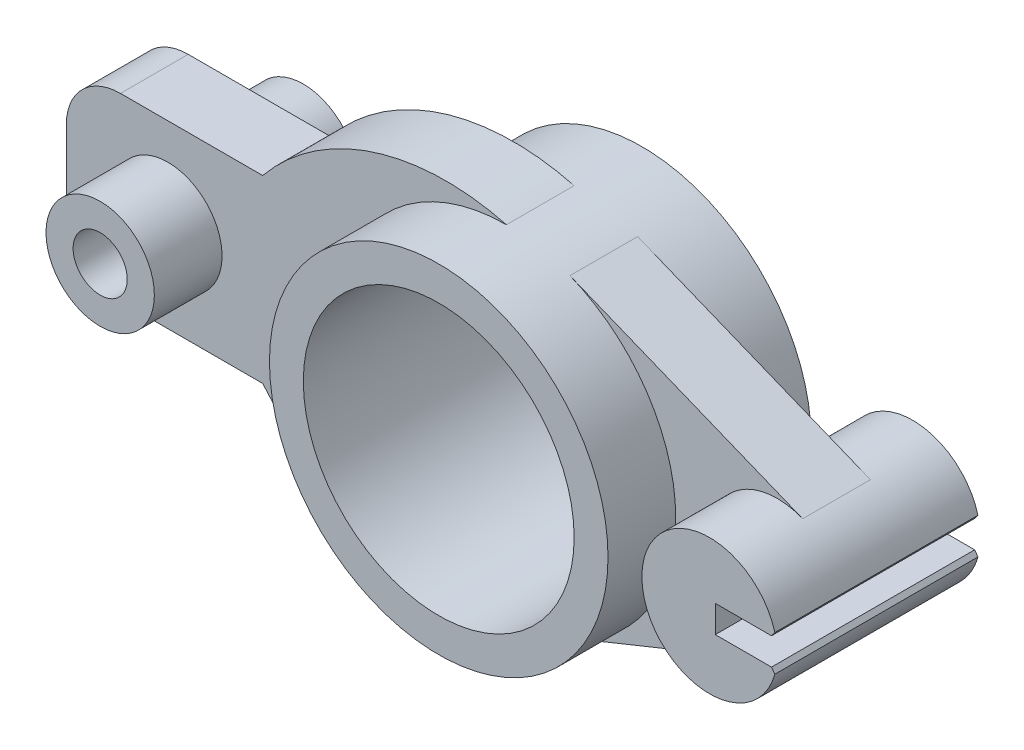
ISO-10303-21;
HEADER;
FILE_DESCRIPTION(('STEP AP214'),'2;1');
FILE_NAME('part.step','',(''),(''),'','','');
FILE_SCHEMA(('AUTOMOTIVE_DESIGN { 1 0 10303 214 1 1 1 1 }'));
ENDSEC;
DATA;
#1=APPLICATION_CONTEXT('core data for automotive mechanical design processes');
#2=APPLICATION_PROTOCOL_DEFINITION('international standard','automotive_design',2000,#1);
#3=PRODUCT_CONTEXT('',#1,'mechanical');
#4=PRODUCT('Part','Part','',(#3));
#5=PRODUCT_RELATED_PRODUCT_CATEGORY('part','',(#4));
#6=PRODUCT_DEFINITION_FORMATION('','',#4);
#7=PRODUCT_DEFINITION_CONTEXT('part definition',#1,'design');
#8=PRODUCT_DEFINITION('design','',#6,#7);
#9=PRODUCT_DEFINITION_SHAPE('','',#8);
#10=(LENGTH_UNIT() NAMED_UNIT(*) SI_UNIT(.MILLI.,.METRE.));
#11=(NAMED_UNIT(*) PLANE_ANGLE_UNIT() SI_UNIT($,.RADIAN.));
#12=(NAMED_UNIT(*) SI_UNIT($,.STERADIAN.) SOLID_ANGLE_UNIT());
#13=UNCERTAINTY_MEASURE_WITH_UNIT(LENGTH_MEASURE(1.E-05),#10,'distance_accuracy_value','');
#14=(GEOMETRIC_REPRESENTATION_CONTEXT(3) GLOBAL_UNCERTAINTY_ASSIGNED_CONTEXT((#13)) GLOBAL_UNIT_ASSIGNED_CONTEXT((#10,
#11,#12)) REPRESENTATION_CONTEXT('',''));
#15=CARTESIAN_POINT('',(0.,0.,0.));
#16=DIRECTION('',(0.,0.,1.));
#17=DIRECTION('',(1.,0.,0.));
#18=AXIS2_PLACEMENT_3D('',#15,#16,#17);
#19=CARTESIAN_POINT('',(0.,0.,15.));
#20=DIRECTION('',(0.,0.,-1.));
#21=DIRECTION('',(-1.,0.,0.));
#22=AXIS2_PLACEMENT_3D('',#19,#20,#21);
#23=CYLINDRICAL_SURFACE('',#22,25.);
#24=CARTESIAN_POINT('',(0.,0.,5.));
#25=DIRECTION('',(0.,0.,-1.));
#26=DIRECTION('',(-1.,0.,0.));
#27=AXIS2_PLACEMENT_3D('',#24,#25,#26);
#28=CIRCLE('',#27,25.);
#29=CARTESIAN_POINT('',(9.37500000000001,23.175620272174,5.));
#30=VERTEX_POINT('',#29);
#31=CARTESIAN_POINT('',(9.37499999999999,-23.175620272174,5.));
#32=VERTEX_POINT('',#31);
#33=EDGE_CURVE('E50',#30,#32,#28,.T.);
#34=ORIENTED_EDGE('',*,*,#33,.F.);
#35=DIRECTION('',(0.,0.,-1.));
#36=VECTOR('',#35,1.);
#37=CARTESIAN_POINT('',(9.37500000000001,23.175620272174,5.));
#38=LINE('',#37,#36);
#39=CARTESIAN_POINT('',(9.37500000000001,23.175620272174,-5.));
#40=VERTEX_POINT('',#39);
#41=EDGE_CURVE('E285',#30,#40,#38,.T.);
#42=ORIENTED_EDGE('',*,*,#41,.T.);
#43=CARTESIAN_POINT('',(0.,0.,-5.));
#44=DIRECTION('',(0.,0.,-1.));
#45=DIRECTION('',(-1.,0.,0.));
#46=AXIS2_PLACEMENT_3D('',#43,#44,#45);
#47=CIRCLE('',#46,25.);
#48=CARTESIAN_POINT('',(9.37500000000001,-23.1756202721739,-5.));
#49=VERTEX_POINT('',#48);
#50=EDGE_CURVE('E323',#40,#49,#47,.T.);
#51=ORIENTED_EDGE('',*,*,#50,.T.);
#52=DIRECTION('',(0.,0.,-1.));
#53=VECTOR('',#52,1.);
#54=CARTESIAN_POINT('',(9.37499999999999,-23.175620272174,5.));
#55=LINE('',#54,#53);
#56=EDGE_CURVE('E295',#32,#49,#55,.T.);
#57=ORIENTED_EDGE('',*,*,#56,.F.);
#58=EDGE_LOOP('',(#34,#42,#51,#57));
#59=FACE_BOUND('',#58,.T.);
#60=CARTESIAN_POINT('',(0.,-25.,-5.));
#61=VERTEX_POINT('',#60);
#62=CARTESIAN_POINT('',(0.,25.,-5.));
#63=VERTEX_POINT('',#62);
#64=EDGE_CURVE('E317',#61,#63,#47,.T.);
#65=ORIENTED_EDGE('',*,*,#64,.T.);
#66=DIRECTION('',(0.,0.,-1.));
#67=VECTOR('',#66,1.);
#68=CARTESIAN_POINT('',(0.,25.,5.));
#69=LINE('',#68,#67);
#70=CARTESIAN_POINT('',(0.,25.,5.));
#71=VERTEX_POINT('',#70);
#72=EDGE_CURVE('E261',#71,#63,#69,.T.);
#73=ORIENTED_EDGE('',*,*,#72,.F.);
#74=CARTESIAN_POINT('',(0.,-25.,5.));
#75=VERTEX_POINT('',#74);
#76=EDGE_CURVE('E322',#75,#71,#28,.T.);
#77=ORIENTED_EDGE('',*,*,#76,.F.);
#78=DIRECTION('',(0.,0.,-1.));
#79=VECTOR('',#78,1.);
#80=CARTESIAN_POINT('',(0.,-25.,5.));
#81=LINE('',#80,#79);
#82=EDGE_CURVE('E294',#75,#61,#81,.T.);
#83=ORIENTED_EDGE('',*,*,#82,.T.);
#84=EDGE_LOOP('',(#65,#73,#77,#83));
#85=FACE_BOUND('',#84,.T.);
#86=CARTESIAN_POINT('',(0.,0.,-15.));
#87=DIRECTION('',(0.,0.,1.));
#88=DIRECTION('',(1.,0.,0.));
#89=AXIS2_PLACEMENT_3D('',#86,#87,#88);
#90=CIRCLE('',#89,25.);
#91=CARTESIAN_POINT('',(25.,0.,-15.));
#92=VERTEX_POINT('',#91);
#93=EDGE_CURVE('E312',#92,#92,#90,.T.);
#94=ORIENTED_EDGE('',*,*,#93,.T.);
#95=EDGE_LOOP('',(#94));
#96=FACE_BOUND('',#95,.T.);
#97=CARTESIAN_POINT('',(0.,0.,15.));
#98=DIRECTION('',(0.,0.,1.));
#99=DIRECTION('',(1.,0.,0.));
#100=AXIS2_PLACEMENT_3D('',#97,#98,#99);
#101=CIRCLE('',#100,25.);
#102=CARTESIAN_POINT('',(25.,0.,15.));
#103=VERTEX_POINT('',#102);
#104=EDGE_CURVE('E316',#103,#103,#101,.T.);
#105=ORIENTED_EDGE('',*,*,#104,.F.);
#106=EDGE_LOOP('',(#105));
#107=FACE_BOUND('',#106,.T.);
#108=ADVANCED_FACE('F39',(#59,#85,#96,#107),#23,.T.);
#109=CARTESIAN_POINT('',(0.,0.,15.));
#110=DIRECTION('',(0.,0.,1.));
#111=DIRECTION('',(1.,0.,0.));
#112=AXIS2_PLACEMENT_3D('',#109,#110,#111);
#113=PLANE('',#112);
#114=CARTESIAN_POINT('',(0.,0.,15.));
#115=DIRECTION('',(0.,0.,1.));
#116=DIRECTION('',(1.,0.,0.));
#117=AXIS2_PLACEMENT_3D('',#114,#115,#116);
#118=CIRCLE('',#117,20.);
#119=CARTESIAN_POINT('',(20.,0.,15.));
#120=VERTEX_POINT('',#119);
#121=EDGE_CURVE('E219',#120,#120,#118,.T.);
#122=ORIENTED_EDGE('',*,*,#121,.F.);
#123=EDGE_LOOP('',(#122));
#124=FACE_BOUND('',#123,.T.);
#125=ORIENTED_EDGE('',*,*,#104,.T.);
#126=EDGE_LOOP('',(#125));
#127=FACE_BOUND('',#126,.T.);
#128=ADVANCED_FACE('F368',(#124,#127),#113,.T.);
#129=CARTESIAN_POINT('',(0.,0.,-15.));
#130=DIRECTION('',(0.,0.,1.));
#131=DIRECTION('',(1.,0.,0.));
#132=AXIS2_PLACEMENT_3D('',#129,#130,#131);
#133=PLANE('',#132);
#134=CARTESIAN_POINT('',(0.,0.,-15.));
#135=DIRECTION('',(0.,0.,1.));
#136=DIRECTION('',(1.,0.,0.));
#137=AXIS2_PLACEMENT_3D('',#134,#135,#136);
#138=CIRCLE('',#137,20.);
#139=CARTESIAN_POINT('',(20.,0.,-15.));
#140=VERTEX_POINT('',#139);
#141=EDGE_CURVE('E216',#140,#140,#138,.T.);
#142=ORIENTED_EDGE('',*,*,#141,.T.);
#143=EDGE_LOOP('',(#142));
#144=FACE_BOUND('',#143,.T.);
#145=ORIENTED_EDGE('',*,*,#93,.F.);
#146=EDGE_LOOP('',(#145));
#147=FACE_BOUND('',#146,.T.);
#148=ADVANCED_FACE('F371',(#144,#147),#133,.F.);
#149=CARTESIAN_POINT('',(-57.,13.2970319871182,5.));
#150=DIRECTION('',(0.,-1.,0.));
#151=DIRECTION('',(1.,0.,0.));
#152=AXIS2_PLACEMENT_3D('',#149,#150,#151);
#153=PLANE('',#152);
#154=DIRECTION('',(-1.,0.,0.));
#155=VECTOR('',#154,1.);
#156=CARTESIAN_POINT('',(-57.,13.2970319871182,-5.));
#157=LINE('',#156,#155);
#158=CARTESIAN_POINT('',(-36.,13.2970319871182,-5.));
#159=VERTEX_POINT('',#158);
#160=CARTESIAN_POINT('',(-57.,13.2970319871182,-5.));
#161=VERTEX_POINT('',#160);
#162=EDGE_CURVE('E264',#159,#161,#157,.T.);
#163=ORIENTED_EDGE('',*,*,#162,.T.);
#164=DIRECTION('',(0.,0.,-1.));
#165=VECTOR('',#164,1.);
#166=CARTESIAN_POINT('',(-57.,13.2970319871182,5.));
#167=LINE('',#166,#165);
#168=CARTESIAN_POINT('',(-57.,13.2970319871182,5.));
#169=VERTEX_POINT('',#168);
#170=EDGE_CURVE('E310',#169,#161,#167,.T.);
#171=ORIENTED_EDGE('',*,*,#170,.F.);
#172=DIRECTION('',(-1.,0.,0.));
#173=VECTOR('',#172,1.);
#174=CARTESIAN_POINT('',(-57.,13.2970319871182,5.));
#175=LINE('',#174,#173);
#176=CARTESIAN_POINT('',(-36.,13.2970319871182,5.));
#177=VERTEX_POINT('',#176);
#178=EDGE_CURVE('E245',#177,#169,#175,.T.);
#179=ORIENTED_EDGE('',*,*,#178,.F.);
#180=DIRECTION('',(0.,0.,-1.));
#181=VECTOR('',#180,1.);
#182=CARTESIAN_POINT('',(-36.,13.2970319871182,5.));
#183=LINE('',#182,#181);
#184=EDGE_CURVE('E315',#177,#159,#183,.T.);
#185=ORIENTED_EDGE('',*,*,#184,.T.);
#186=EDGE_LOOP('',(#163,#171,#179,#185));
#187=FACE_BOUND('',#186,.T.);
#188=ADVANCED_FACE('F378',(#187),#153,.F.);
#189=CARTESIAN_POINT('',(-57.,5.29703198711818,5.));
#190=DIRECTION('',(0.,0.,-1.));
#191=DIRECTION('',(-1.,0.,0.));
#192=AXIS2_PLACEMENT_3D('',#189,#190,#191);
#193=CYLINDRICAL_SURFACE('',#192,8.);
#194=CARTESIAN_POINT('',(-57.,5.29703198711818,-5.));
#195=DIRECTION('',(0.,0.,1.));
#196=DIRECTION('',(1.,0.,0.));
#197=AXIS2_PLACEMENT_3D('',#194,#195,#196);
#198=CIRCLE('',#197,8.);
#199=CARTESIAN_POINT('',(-65.,5.29703198711818,-5.));
#200=VERTEX_POINT('',#199);
#201=EDGE_CURVE('E270',#161,#200,#198,.T.);
#202=ORIENTED_EDGE('',*,*,#201,.T.);
#203=DIRECTION('',(0.,0.,-1.));
#204=VECTOR('',#203,1.);
#205=CARTESIAN_POINT('',(-65.,5.29703198711818,5.));
#206=LINE('',#205,#204);
#207=CARTESIAN_POINT('',(-65.,5.29703198711818,5.));
#208=VERTEX_POINT('',#207);
#209=EDGE_CURVE('E308',#208,#200,#206,.T.);
#210=ORIENTED_EDGE('',*,*,#209,.F.);
#211=CARTESIAN_POINT('',(-57.,5.29703198711818,5.));
#212=DIRECTION('',(0.,0.,1.));
#213=DIRECTION('',(1.,0.,0.));
#214=AXIS2_PLACEMENT_3D('',#211,#212,#213);
#215=CIRCLE('',#214,8.);
#216=EDGE_CURVE('E248',#169,#208,#215,.T.);
#217=ORIENTED_EDGE('',*,*,#216,.F.);
#218=ORIENTED_EDGE('',*,*,#170,.T.);
#219=EDGE_LOOP('',(#202,#210,#217,#218));
#220=FACE_BOUND('',#219,.T.);
#221=ADVANCED_FACE('F383',(#220),#193,.T.);
#222=CARTESIAN_POINT('',(-65.,-5.29703198711821,5.));
#223=DIRECTION('',(1.,0.,0.));
#224=DIRECTION('',(0.,0.,-1.));
#225=AXIS2_PLACEMENT_3D('',#222,#223,#224);
#226=PLANE('',#225);
#227=DIRECTION('',(0.,-1.,0.));
#228=VECTOR('',#227,1.);
#229=CARTESIAN_POINT('',(-65.,-5.29703198711821,-5.));
#230=LINE('',#229,#228);
#231=CARTESIAN_POINT('',(-65.,-5.29703198711821,-5.));
#232=VERTEX_POINT('',#231);
#233=EDGE_CURVE('E267',#200,#232,#230,.T.);
#234=ORIENTED_EDGE('',*,*,#233,.T.);
#235=DIRECTION('',(0.,0.,-1.));
#236=VECTOR('',#235,1.);
#237=CARTESIAN_POINT('',(-65.,-5.29703198711821,5.));
#238=LINE('',#237,#236);
#239=CARTESIAN_POINT('',(-65.,-5.29703198711821,5.));
#240=VERTEX_POINT('',#239);
#241=EDGE_CURVE('E302',#240,#232,#238,.T.);
#242=ORIENTED_EDGE('',*,*,#241,.F.);
#243=DIRECTION('',(0.,-1.,0.));
#244=VECTOR('',#243,1.);
#245=CARTESIAN_POINT('',(-65.,-5.29703198711821,5.));
#246=LINE('',#245,#244);
#247=EDGE_CURVE('E247',#208,#240,#246,.T.);
#248=ORIENTED_EDGE('',*,*,#247,.F.);
#249=ORIENTED_EDGE('',*,*,#209,.T.);
#250=EDGE_LOOP('',(#234,#242,#248,#249));
#251=FACE_BOUND('',#250,.T.);
#252=ADVANCED_FACE('F389',(#251),#226,.F.);
#253=CARTESIAN_POINT('',(-57.,-5.29703198711821,5.));
#254=DIRECTION('',(0.,0.,-1.));
#255=DIRECTION('',(-1.,0.,0.));
#256=AXIS2_PLACEMENT_3D('',#253,#254,#255);
#257=CYLINDRICAL_SURFACE('',#256,8.);
#258=CARTESIAN_POINT('',(-57.,-5.29703198711821,-5.));
#259=DIRECTION('',(0.,0.,1.));
#260=DIRECTION('',(-1.,0.,0.));
#261=AXIS2_PLACEMENT_3D('',#258,#259,#260);
#262=CIRCLE('',#261,8.);
#263=CARTESIAN_POINT('',(-57.,-13.2970319871182,-5.));
#264=VERTEX_POINT('',#263);
#265=EDGE_CURVE('E271',#232,#264,#262,.T.);
#266=ORIENTED_EDGE('',*,*,#265,.T.);
#267=DIRECTION('',(0.,0.,-1.));
#268=VECTOR('',#267,1.);
#269=CARTESIAN_POINT('',(-57.,-13.2970319871182,5.));
#270=LINE('',#269,#268);
#271=CARTESIAN_POINT('',(-57.,-13.2970319871182,5.));
#272=VERTEX_POINT('',#271);
#273=EDGE_CURVE('E298',#272,#264,#270,.T.);
#274=ORIENTED_EDGE('',*,*,#273,.F.);
#275=CARTESIAN_POINT('',(-57.,-5.29703198711821,5.));
#276=DIRECTION('',(0.,0.,1.));
#277=DIRECTION('',(-1.,0.,0.));
#278=AXIS2_PLACEMENT_3D('',#275,#276,#277);
#279=CIRCLE('',#278,8.);
#280=EDGE_CURVE('E246',#240,#272,#279,.T.);
#281=ORIENTED_EDGE('',*,*,#280,.F.);
#282=ORIENTED_EDGE('',*,*,#241,.T.);
#283=EDGE_LOOP('',(#266,#274,#281,#282));
#284=FACE_BOUND('',#283,.T.);
#285=ADVANCED_FACE('F394',(#284),#257,.T.);
#286=CARTESIAN_POINT('',(-57.,-13.2970319871182,5.));
#287=DIRECTION('',(0.,1.,0.));
#288=DIRECTION('',(-1.,0.,0.));
#289=AXIS2_PLACEMENT_3D('',#286,#287,#288);
#290=PLANE('',#289);
#291=DIRECTION('',(1.,0.,0.));
#292=VECTOR('',#291,1.);
#293=CARTESIAN_POINT('',(-57.,-13.2970319871182,-5.));
#294=LINE('',#293,#292);
#295=CARTESIAN_POINT('',(-36.,-13.2970319871182,-5.));
#296=VERTEX_POINT('',#295);
#297=EDGE_CURVE('E272',#264,#296,#294,.T.);
#298=ORIENTED_EDGE('',*,*,#297,.T.);
#299=DIRECTION('',(0.,0.,-1.));
#300=VECTOR('',#299,1.);
#301=CARTESIAN_POINT('',(-36.,-13.2970319871182,5.));
#302=LINE('',#301,#300);
#303=CARTESIAN_POINT('',(-36.,-13.2970319871182,5.));
#304=VERTEX_POINT('',#303);
#305=EDGE_CURVE('E299',#304,#296,#302,.T.);
#306=ORIENTED_EDGE('',*,*,#305,.F.);
#307=DIRECTION('',(1.,0.,0.));
#308=VECTOR('',#307,1.);
#309=CARTESIAN_POINT('',(-57.,-13.2970319871182,5.));
#310=LINE('',#309,#308);
#311=EDGE_CURVE('E252',#272,#304,#310,.T.);
#312=ORIENTED_EDGE('',*,*,#311,.F.);
#313=ORIENTED_EDGE('',*,*,#273,.T.);
#314=EDGE_LOOP('',(#298,#306,#312,#313));
#315=FACE_BOUND('',#314,.T.);
#316=ADVANCED_FACE('F361',(#315),#290,.F.);
#317=CARTESIAN_POINT('',(-8.89817396997828,-8.85000000000002,5.));
#318=DIRECTION('',(0.,0.,-1.));
#319=DIRECTION('',(-1.,0.,0.));
#320=AXIS2_PLACEMENT_3D('',#317,#318,#319);
#321=PLANE('',#320);
#322=CARTESIAN_POINT('',(-50.,0.,5.));
#323=DIRECTION('',(0.,0.,-1.));
#324=DIRECTION('',(-1.,0.,0.));
#325=AXIS2_PLACEMENT_3D('',#322,#323,#324);
#326=CIRCLE('',#325,7.99999999999999);
#327=CARTESIAN_POINT('',(-58.,0.,5.));
#328=VERTEX_POINT('',#327);
#329=EDGE_CURVE('E11',#328,#328,#326,.F.);
#330=ORIENTED_EDGE('',*,*,#329,.F.);
#331=EDGE_LOOP('',(#330));
#332=FACE_BOUND('',#331,.T.);
#333=CARTESIAN_POINT('',(-8.89817396997828,8.85,5.));
#334=DIRECTION('',(0.,0.,1.));
#335=DIRECTION('',(1.,0.,0.));
#336=AXIS2_PLACEMENT_3D('',#333,#334,#335);
#337=CIRCLE('',#336,35.);
#338=EDGE_CURVE('E255',#304,#75,#337,.T.);
#339=ORIENTED_EDGE('',*,*,#338,.T.);
#340=ORIENTED_EDGE('',*,*,#76,.T.);
#341=CARTESIAN_POINT('',(-8.89817396997828,-8.85000000000002,5.));
#342=DIRECTION('',(0.,0.,1.));
#343=DIRECTION('',(-1.,0.,0.));
#344=AXIS2_PLACEMENT_3D('',#341,#342,#343);
#345=CIRCLE('',#344,35.);
#346=EDGE_CURVE('E238',#71,#177,#345,.T.);
#347=ORIENTED_EDGE('',*,*,#346,.T.);
#348=ORIENTED_EDGE('',*,*,#178,.T.);
#349=ORIENTED_EDGE('',*,*,#216,.T.);
#350=ORIENTED_EDGE('',*,*,#247,.T.);
#351=ORIENTED_EDGE('',*,*,#280,.T.);
#352=ORIENTED_EDGE('',*,*,#311,.T.);
#353=EDGE_LOOP('',(#339,#340,#347,#348,#349,#350,#351,#352));
#354=FACE_BOUND('',#353,.T.);
#355=ADVANCED_FACE('F352',(#332,#354),#321,.F.);
#356=CARTESIAN_POINT('',(-8.89817396997828,-8.85000000000002,-5.));
#357=DIRECTION('',(0.,0.,-1.));
#358=DIRECTION('',(-1.,0.,0.));
#359=AXIS2_PLACEMENT_3D('',#356,#357,#358);
#360=PLANE('',#359);
#361=CARTESIAN_POINT('',(-50.,0.,-5.));
#362=DIRECTION('',(0.,0.,-1.));
#363=DIRECTION('',(-1.,0.,0.));
#364=AXIS2_PLACEMENT_3D('',#361,#362,#363);
#365=CIRCLE('',#364,7.99999999999999);
#366=CARTESIAN_POINT('',(-58.,0.,-5.));
#367=VERTEX_POINT('',#366);
#368=EDGE_CURVE('E45',#367,#367,#365,.F.);
#369=ORIENTED_EDGE('',*,*,#368,.T.);
#370=EDGE_LOOP('',(#369));
#371=FACE_BOUND('',#370,.T.);
#372=ORIENTED_EDGE('',*,*,#64,.F.);
#373=CARTESIAN_POINT('',(-8.89817396997828,8.85,-5.));
#374=DIRECTION('',(0.,0.,1.));
#375=DIRECTION('',(1.,0.,0.));
#376=AXIS2_PLACEMENT_3D('',#373,#374,#375);
#377=CIRCLE('',#376,35.);
#378=EDGE_CURVE('E274',#296,#61,#377,.T.);
#379=ORIENTED_EDGE('',*,*,#378,.F.);
#380=ORIENTED_EDGE('',*,*,#297,.F.);
#381=ORIENTED_EDGE('',*,*,#265,.F.);
#382=ORIENTED_EDGE('',*,*,#233,.F.);
#383=ORIENTED_EDGE('',*,*,#201,.F.);
#384=ORIENTED_EDGE('',*,*,#162,.F.);
#385=CARTESIAN_POINT('',(-8.89817396997828,-8.85000000000002,-5.));
#386=DIRECTION('',(0.,0.,1.));
#387=DIRECTION('',(-1.,0.,0.));
#388=AXIS2_PLACEMENT_3D('',#385,#386,#387);
#389=CIRCLE('',#388,35.);
#390=EDGE_CURVE('E265',#63,#159,#389,.T.);
#391=ORIENTED_EDGE('',*,*,#390,.F.);
#392=EDGE_LOOP('',(#372,#379,#380,#381,#382,#383,#384,#391));
#393=FACE_BOUND('',#392,.T.);
#394=ADVANCED_FACE('F359',(#371,#393),#360,.T.);
#395=CARTESIAN_POINT('',(-8.89817396997828,8.85,5.));
#396=DIRECTION('',(0.,0.,-1.));
#397=DIRECTION('',(-1.,0.,0.));
#398=AXIS2_PLACEMENT_3D('',#395,#396,#397);
#399=CYLINDRICAL_SURFACE('',#398,35.);
#400=ORIENTED_EDGE('',*,*,#378,.T.);
#401=ORIENTED_EDGE('',*,*,#82,.F.);
#402=ORIENTED_EDGE('',*,*,#338,.F.);
#403=ORIENTED_EDGE('',*,*,#305,.T.);
#404=EDGE_LOOP('',(#400,#401,#402,#403));
#405=FACE_BOUND('',#404,.T.);
#406=ADVANCED_FACE('F357',(#405),#399,.T.);
#407=CARTESIAN_POINT('',(-8.89817396997828,-8.85000000000002,5.));
#408=DIRECTION('',(0.,0.,-1.));
#409=DIRECTION('',(-1.,0.,0.));
#410=AXIS2_PLACEMENT_3D('',#407,#408,#409);
#411=CYLINDRICAL_SURFACE('',#410,35.);
#412=ORIENTED_EDGE('',*,*,#390,.T.);
#413=ORIENTED_EDGE('',*,*,#184,.F.);
#414=ORIENTED_EDGE('',*,*,#346,.F.);
#415=ORIENTED_EDGE('',*,*,#72,.T.);
#416=EDGE_LOOP('',(#412,#413,#414,#415));
#417=FACE_BOUND('',#416,.T.);
#418=ADVANCED_FACE('F349',(#417),#411,.T.);
#419=CARTESIAN_POINT('',(40.,0.,5.));
#420=DIRECTION('',(0.,0.,-1.));
#421=DIRECTION('',(-1.,0.,0.));
#422=AXIS2_PLACEMENT_3D('',#419,#420,#421);
#423=CIRCLE('',#422,9.99999999999999);
#424=CARTESIAN_POINT('',(43.75,9.27024810886957,5.));
#425=VERTEX_POINT('',#424);
#426=CARTESIAN_POINT('',(43.75,-9.27024810886957,5.));
#427=VERTEX_POINT('',#426);
#428=EDGE_CURVE('E233',#425,#427,#423,.F.);
#429=ORIENTED_EDGE('',*,*,#428,.F.);
#430=DIRECTION('',(-0.927024810886958,0.375,0.));
#431=VECTOR('',#430,1.);
#432=CARTESIAN_POINT('',(9.37500000000001,23.175620272174,5.));
#433=LINE('',#432,#431);
#434=EDGE_CURVE('E259',#425,#30,#433,.T.);
#435=ORIENTED_EDGE('',*,*,#434,.T.);
#436=ORIENTED_EDGE('',*,*,#33,.T.);
#437=DIRECTION('',(0.927024810886958,0.375,0.));
#438=VECTOR('',#437,1.);
#439=CARTESIAN_POINT('',(9.37500000000001,-23.175620272174,5.));
#440=LINE('',#439,#438);
#441=EDGE_CURVE('E258',#32,#427,#440,.T.);
#442=ORIENTED_EDGE('',*,*,#441,.T.);
#443=EDGE_LOOP('',(#429,#435,#436,#442));
#444=FACE_BOUND('',#443,.T.);
#445=ADVANCED_FACE('F350',(#444),#321,.F.);
#446=DIRECTION('',(-0.927024810886958,0.375,0.));
#447=VECTOR('',#446,1.);
#448=CARTESIAN_POINT('',(9.37500000000001,23.175620272174,-5.));
#449=LINE('',#448,#447);
#450=CARTESIAN_POINT('',(43.75,9.27024810886957,-5.));
#451=VERTEX_POINT('',#450);
#452=EDGE_CURVE('E241',#451,#40,#449,.T.);
#453=ORIENTED_EDGE('',*,*,#452,.F.);
#454=CARTESIAN_POINT('',(40.,0.,-5.));
#455=DIRECTION('',(0.,0.,-1.));
#456=DIRECTION('',(-1.,0.,0.));
#457=AXIS2_PLACEMENT_3D('',#454,#455,#456);
#458=CIRCLE('',#457,9.99999999999999);
#459=CARTESIAN_POINT('',(43.75,-9.27024810886957,-5.));
#460=VERTEX_POINT('',#459);
#461=EDGE_CURVE('E229',#451,#460,#458,.F.);
#462=ORIENTED_EDGE('',*,*,#461,.T.);
#463=DIRECTION('',(0.927024810886958,0.375,0.));
#464=VECTOR('',#463,1.);
#465=CARTESIAN_POINT('',(9.37500000000001,-23.175620272174,-5.));
#466=LINE('',#465,#464);
#467=EDGE_CURVE('E65',#49,#460,#466,.T.);
#468=ORIENTED_EDGE('',*,*,#467,.F.);
#469=ORIENTED_EDGE('',*,*,#50,.F.);
#470=EDGE_LOOP('',(#453,#462,#468,#469));
#471=FACE_BOUND('',#470,.T.);
#472=ADVANCED_FACE('F333',(#471),#360,.T.);
#473=CARTESIAN_POINT('',(9.37500000000001,-23.175620272174,5.));
#474=DIRECTION('',(-0.375,0.927024810886958,0.));
#475=DIRECTION('',(-0.927024810886958,-0.375,0.));
#476=AXIS2_PLACEMENT_3D('',#473,#474,#475);
#477=PLANE('',#476);
#478=ORIENTED_EDGE('',*,*,#467,.T.);
#479=DIRECTION('',(0.,0.,-1.));
#480=VECTOR('',#479,1.);
#481=CARTESIAN_POINT('',(43.75,-9.27024810886957,5.));
#482=LINE('',#481,#480);
#483=EDGE_CURVE('E290',#427,#460,#482,.T.);
#484=ORIENTED_EDGE('',*,*,#483,.F.);
#485=ORIENTED_EDGE('',*,*,#441,.F.);
#486=ORIENTED_EDGE('',*,*,#56,.T.);
#487=EDGE_LOOP('',(#478,#484,#485,#486));
#488=FACE_BOUND('',#487,.T.);
#489=ADVANCED_FACE('F345',(#488),#477,.F.);
#490=CARTESIAN_POINT('',(40.,0.,5.));
#491=DIRECTION('',(0.,0.,-1.));
#492=DIRECTION('',(-1.,0.,0.));
#493=AXIS2_PLACEMENT_3D('',#490,#491,#492);
#494=CYLINDRICAL_SURFACE('',#493,9.99999999999999);
#495=ORIENTED_EDGE('',*,*,#483,.T.);
#496=ORIENTED_EDGE('',*,*,#461,.F.);
#497=DIRECTION('',(0.,0.,-1.));
#498=VECTOR('',#497,1.);
#499=CARTESIAN_POINT('',(43.75,9.27024810886957,5.));
#500=LINE('',#499,#498);
#501=EDGE_CURVE('E288',#425,#451,#500,.T.);
#502=ORIENTED_EDGE('',*,*,#501,.F.);
#503=ORIENTED_EDGE('',*,*,#428,.T.);
#504=EDGE_LOOP('',(#495,#496,#502,#503));
#505=FACE_BOUND('',#504,.T.);
#506=CARTESIAN_POINT('',(40.,0.,15.));
#507=DIRECTION('',(0.,0.,1.));
#508=DIRECTION('',(1.,0.,0.));
#509=AXIS2_PLACEMENT_3D('',#506,#507,#508);
#510=CIRCLE('',#509,9.99999999999999);
#511=CARTESIAN_POINT('',(49.6387576153315,2.6635224108102,15.));
#512=VERTEX_POINT('',#511);
#513=CARTESIAN_POINT('',(49.6387576153315,-2.6635224108102,15.));
#514=VERTEX_POINT('',#513);
#515=EDGE_CURVE('E221',#512,#514,#510,.T.);
#516=ORIENTED_EDGE('',*,*,#515,.F.);
#517=DIRECTION('',(0.,0.,1.));
#518=VECTOR('',#517,1.);
#519=CARTESIAN_POINT('',(49.6387576153315,2.6635224108102,-15.));
#520=LINE('',#519,#518);
#521=CARTESIAN_POINT('',(49.6387576153315,2.6635224108102,-15.));
#522=VERTEX_POINT('',#521);
#523=EDGE_CURVE('E208',#522,#512,#520,.T.);
#524=ORIENTED_EDGE('',*,*,#523,.F.);
#525=CARTESIAN_POINT('',(40.,0.,-15.));
#526=DIRECTION('',(0.,0.,1.));
#527=DIRECTION('',(1.,0.,0.));
#528=AXIS2_PLACEMENT_3D('',#525,#526,#527);
#529=CIRCLE('',#528,9.99999999999999);
#530=CARTESIAN_POINT('',(49.6387576153315,-2.6635224108102,-15.));
#531=VERTEX_POINT('',#530);
#532=EDGE_CURVE('E218',#522,#531,#529,.T.);
#533=ORIENTED_EDGE('',*,*,#532,.T.);
#534=DIRECTION('',(0.,0.,1.));
#535=VECTOR('',#534,1.);
#536=CARTESIAN_POINT('',(49.6387576153315,-2.6635224108102,-15.));
#537=LINE('',#536,#535);
#538=EDGE_CURVE('E209',#531,#514,#537,.T.);
#539=ORIENTED_EDGE('',*,*,#538,.T.);
#540=EDGE_LOOP('',(#516,#524,#533,#539));
#541=FACE_BOUND('',#540,.T.);
#542=ADVANCED_FACE('F343',(#505,#541),#494,.T.);
#543=CARTESIAN_POINT('',(9.37500000000001,23.175620272174,5.));
#544=DIRECTION('',(-0.375,-0.927024810886958,0.));
#545=DIRECTION('',(0.927024810886958,-0.375,0.));
#546=AXIS2_PLACEMENT_3D('',#543,#544,#545);
#547=PLANE('',#546);
#548=ORIENTED_EDGE('',*,*,#452,.T.);
#549=ORIENTED_EDGE('',*,*,#41,.F.);
#550=ORIENTED_EDGE('',*,*,#434,.F.);
#551=ORIENTED_EDGE('',*,*,#501,.T.);
#552=EDGE_LOOP('',(#548,#549,#550,#551));
#553=FACE_BOUND('',#552,.T.);
#554=ADVANCED_FACE('F339',(#553),#547,.F.);
#555=CARTESIAN_POINT('',(-50.,0.,-15.));
#556=DIRECTION('',(0.,0.,1.));
#557=DIRECTION('',(1.,0.,0.));
#558=AXIS2_PLACEMENT_3D('',#555,#556,#557);
#559=PLANE('',#558);
#560=CARTESIAN_POINT('',(-50.,0.,-15.));
#561=DIRECTION('',(0.,0.,1.));
#562=DIRECTION('',(1.,0.,0.));
#563=AXIS2_PLACEMENT_3D('',#560,#561,#562);
#564=CIRCLE('',#563,4.00000000000001);
#565=CARTESIAN_POINT('',(-46.,0.,-15.));
#566=VERTEX_POINT('',#565);
#567=EDGE_CURVE('E224',#566,#566,#564,.T.);
#568=ORIENTED_EDGE('',*,*,#567,.T.);
#569=EDGE_LOOP('',(#568));
#570=FACE_BOUND('',#569,.T.);
#571=CARTESIAN_POINT('',(-50.,0.,-15.));
#572=DIRECTION('',(0.,0.,1.));
#573=DIRECTION('',(1.,0.,0.));
#574=AXIS2_PLACEMENT_3D('',#571,#572,#573);
#575=CIRCLE('',#574,7.99999999999999);
#576=CARTESIAN_POINT('',(-42.,0.,-15.));
#577=VERTEX_POINT('',#576);
#578=EDGE_CURVE('E235',#577,#577,#575,.T.);
#579=ORIENTED_EDGE('',*,*,#578,.F.);
#580=EDGE_LOOP('',(#579));
#581=FACE_BOUND('',#580,.T.);
#582=ADVANCED_FACE('F410',(#570,#581),#559,.F.);
#583=CARTESIAN_POINT('',(-50.,0.,15.));
#584=DIRECTION('',(0.,0.,-1.));
#585=DIRECTION('',(-1.,0.,0.));
#586=AXIS2_PLACEMENT_3D('',#583,#584,#585);
#587=CYLINDRICAL_SURFACE('',#586,7.99999999999999);
#588=ORIENTED_EDGE('',*,*,#368,.F.);
#589=EDGE_LOOP('',(#588));
#590=FACE_BOUND('',#589,.T.);
#591=ORIENTED_EDGE('',*,*,#578,.T.);
#592=EDGE_LOOP('',(#591));
#593=FACE_BOUND('',#592,.T.);
#594=ADVANCED_FACE('F439',(#590,#593),#587,.T.);
#595=CARTESIAN_POINT('',(-50.,0.,15.));
#596=DIRECTION('',(0.,0.,1.));
#597=DIRECTION('',(1.,0.,0.));
#598=AXIS2_PLACEMENT_3D('',#595,#596,#597);
#599=CIRCLE('',#598,7.99999999999999);
#600=CARTESIAN_POINT('',(-42.,0.,15.));
#601=VERTEX_POINT('',#600);
#602=EDGE_CURVE('E231',#601,#601,#599,.T.);
#603=ORIENTED_EDGE('',*,*,#602,.F.);
#604=EDGE_LOOP('',(#603));
#605=FACE_BOUND('',#604,.T.);
#606=ORIENTED_EDGE('',*,*,#329,.T.);
#607=EDGE_LOOP('',(#606));
#608=FACE_BOUND('',#607,.T.);
#609=ADVANCED_FACE('F444',(#605,#608),#587,.T.);
#610=CARTESIAN_POINT('',(-50.,0.,15.));
#611=DIRECTION('',(0.,0.,1.));
#612=DIRECTION('',(1.,0.,0.));
#613=AXIS2_PLACEMENT_3D('',#610,#611,#612);
#614=PLANE('',#613);
#615=CARTESIAN_POINT('',(-50.,0.,15.));
#616=DIRECTION('',(0.,0.,1.));
#617=DIRECTION('',(1.,0.,0.));
#618=AXIS2_PLACEMENT_3D('',#615,#616,#617);
#619=CIRCLE('',#618,4.00000000000001);
#620=CARTESIAN_POINT('',(-46.,0.,15.));
#621=VERTEX_POINT('',#620);
#622=EDGE_CURVE('E193',#621,#621,#619,.T.);
#623=ORIENTED_EDGE('',*,*,#622,.F.);
#624=EDGE_LOOP('',(#623));
#625=FACE_BOUND('',#624,.T.);
#626=ORIENTED_EDGE('',*,*,#602,.T.);
#627=EDGE_LOOP('',(#626));
#628=FACE_BOUND('',#627,.T.);
#629=ADVANCED_FACE('F455',(#625,#628),#614,.T.);
#630=CARTESIAN_POINT('',(40.,0.,-15.));
#631=DIRECTION('',(0.,0.,1.));
#632=DIRECTION('',(1.,0.,0.));
#633=AXIS2_PLACEMENT_3D('',#630,#631,#632);
#634=PLANE('',#633);
#635=ORIENTED_EDGE('',*,*,#532,.F.);
#636=DIRECTION('',(-0.601815023152049,-0.798635510047292,0.));
#637=VECTOR('',#636,1.);
#638=CARTESIAN_POINT('',(49.1387576153315,2.,-15.));
#639=LINE('',#638,#637);
#640=CARTESIAN_POINT('',(49.1387576153315,2.,-15.));
#641=VERTEX_POINT('',#640);
#642=EDGE_CURVE('E175',#522,#641,#639,.T.);
#643=ORIENTED_EDGE('',*,*,#642,.T.);
#644=DIRECTION('',(-1.,0.,0.));
#645=VECTOR('',#644,1.);
#646=CARTESIAN_POINT('',(40.8450517285068,2.,-15.));
#647=LINE('',#646,#645);
#648=CARTESIAN_POINT('',(40.8450517285068,2.,-15.));
#649=VERTEX_POINT('',#648);
#650=EDGE_CURVE('E170',#641,#649,#647,.T.);
#651=ORIENTED_EDGE('',*,*,#650,.T.);
#652=DIRECTION('',(0.,-1.,0.));
#653=VECTOR('',#652,1.);
#654=CARTESIAN_POINT('',(40.8450517285068,2.,-15.));
#655=LINE('',#654,#653);
#656=CARTESIAN_POINT('',(40.8450517285068,-2.,-15.));
#657=VERTEX_POINT('',#656);
#658=EDGE_CURVE('E178',#649,#657,#655,.T.);
#659=ORIENTED_EDGE('',*,*,#658,.T.);
#660=DIRECTION('',(1.,0.,0.));
#661=VECTOR('',#660,1.);
#662=CARTESIAN_POINT('',(40.8450517285068,-2.,-15.));
#663=LINE('',#662,#661);
#664=CARTESIAN_POINT('',(49.1450517285068,-2.,-15.));
#665=VERTEX_POINT('',#664);
#666=EDGE_CURVE('E182',#657,#665,#663,.T.);
#667=ORIENTED_EDGE('',*,*,#666,.T.);
#668=DIRECTION('',(0.596949889654469,-0.80227852348266,0.));
#669=VECTOR('',#668,1.);
#670=CARTESIAN_POINT('',(49.1450517285068,-2.,-15.));
#671=LINE('',#670,#669);
#672=EDGE_CURVE('E191',#665,#531,#671,.T.);
#673=ORIENTED_EDGE('',*,*,#672,.T.);
#674=EDGE_LOOP('',(#635,#643,#651,#659,#667,#673));
#675=FACE_BOUND('',#674,.T.);
#676=ADVANCED_FACE('F184',(#675),#634,.F.);
#677=CARTESIAN_POINT('',(40.,0.,15.));
#678=DIRECTION('',(0.,0.,1.));
#679=DIRECTION('',(1.,0.,0.));
#680=AXIS2_PLACEMENT_3D('',#677,#678,#679);
#681=PLANE('',#680);
#682=DIRECTION('',(-0.601815023152049,-0.798635510047292,0.));
#683=VECTOR('',#682,1.);
#684=CARTESIAN_POINT('',(49.1387576153315,2.,15.));
#685=LINE('',#684,#683);
#686=CARTESIAN_POINT('',(49.1387576153315,2.,15.));
#687=VERTEX_POINT('',#686);
#688=EDGE_CURVE('E183',#512,#687,#685,.T.);
#689=ORIENTED_EDGE('',*,*,#688,.F.);
#690=ORIENTED_EDGE('',*,*,#515,.T.);
#691=DIRECTION('',(0.596949889654469,-0.80227852348266,0.));
#692=VECTOR('',#691,1.);
#693=CARTESIAN_POINT('',(49.1450517285068,-2.,15.));
#694=LINE('',#693,#692);
#695=CARTESIAN_POINT('',(49.1450517285068,-2.,15.));
#696=VERTEX_POINT('',#695);
#697=EDGE_CURVE('E190',#696,#514,#694,.T.);
#698=ORIENTED_EDGE('',*,*,#697,.F.);
#699=DIRECTION('',(1.,0.,0.));
#700=VECTOR('',#699,1.);
#701=CARTESIAN_POINT('',(40.8450517285068,-2.,15.));
#702=LINE('',#701,#700);
#703=CARTESIAN_POINT('',(40.8450517285068,-2.,15.));
#704=VERTEX_POINT('',#703);
#705=EDGE_CURVE('E205',#704,#696,#702,.T.);
#706=ORIENTED_EDGE('',*,*,#705,.F.);
#707=DIRECTION('',(0.,-1.,0.));
#708=VECTOR('',#707,1.);
#709=CARTESIAN_POINT('',(40.8450517285068,2.,15.));
#710=LINE('',#709,#708);
#711=CARTESIAN_POINT('',(40.8450517285068,2.,15.));
#712=VERTEX_POINT('',#711);
#713=EDGE_CURVE('E199',#712,#704,#710,.T.);
#714=ORIENTED_EDGE('',*,*,#713,.F.);
#715=DIRECTION('',(-1.,0.,0.));
#716=VECTOR('',#715,1.);
#717=CARTESIAN_POINT('',(40.8450517285068,2.,15.));
#718=LINE('',#717,#716);
#719=EDGE_CURVE('E54',#687,#712,#718,.T.);
#720=ORIENTED_EDGE('',*,*,#719,.F.);
#721=EDGE_LOOP('',(#689,#690,#698,#706,#714,#720));
#722=FACE_BOUND('',#721,.T.);
#723=ADVANCED_FACE('F459',(#722),#681,.T.);
#724=CARTESIAN_POINT('',(40.8450517285068,2.,-15.));
#725=DIRECTION('',(0.,1.,0.));
#726=DIRECTION('',(0.,0.,1.));
#727=AXIS2_PLACEMENT_3D('',#724,#725,#726);
#728=PLANE('',#727);
#729=ORIENTED_EDGE('',*,*,#719,.T.);
#730=DIRECTION('',(0.,0.,1.));
#731=VECTOR('',#730,1.);
#732=CARTESIAN_POINT('',(40.8450517285068,2.,-15.));
#733=LINE('',#732,#731);
#734=EDGE_CURVE('E162',#649,#712,#733,.T.);
#735=ORIENTED_EDGE('',*,*,#734,.F.);
#736=ORIENTED_EDGE('',*,*,#650,.F.);
#737=DIRECTION('',(0.,0.,1.));
#738=VECTOR('',#737,1.);
#739=CARTESIAN_POINT('',(49.1387576153315,2.,-15.));
#740=LINE('',#739,#738);
#741=EDGE_CURVE('E206',#641,#687,#740,.T.);
#742=ORIENTED_EDGE('',*,*,#741,.T.);
#743=EDGE_LOOP('',(#729,#735,#736,#742));
#744=FACE_BOUND('',#743,.T.);
#745=ADVANCED_FACE('F164',(#744),#728,.F.);
#746=CARTESIAN_POINT('',(49.1387576153315,2.,-15.));
#747=DIRECTION('',(-0.798635510047292,0.601815023152049,0.));
#748=DIRECTION('',(-0.601815023152049,-0.798635510047292,0.));
#749=AXIS2_PLACEMENT_3D('',#746,#747,#748);
#750=PLANE('',#749);
#751=ORIENTED_EDGE('',*,*,#688,.T.);
#752=ORIENTED_EDGE('',*,*,#741,.F.);
#753=ORIENTED_EDGE('',*,*,#642,.F.);
#754=ORIENTED_EDGE('',*,*,#523,.T.);
#755=EDGE_LOOP('',(#751,#752,#753,#754));
#756=FACE_BOUND('',#755,.T.);
#757=ADVANCED_FACE('F466',(#756),#750,.F.);
#758=CARTESIAN_POINT('',(49.1450517285068,-2.,-15.));
#759=DIRECTION('',(-0.80227852348266,-0.596949889654469,0.));
#760=DIRECTION('',(0.596949889654469,-0.80227852348266,0.));
#761=AXIS2_PLACEMENT_3D('',#758,#759,#760);
#762=PLANE('',#761);
#763=ORIENTED_EDGE('',*,*,#697,.T.);
#764=ORIENTED_EDGE('',*,*,#538,.F.);
#765=ORIENTED_EDGE('',*,*,#672,.F.);
#766=DIRECTION('',(0.,0.,1.));
#767=VECTOR('',#766,1.);
#768=CARTESIAN_POINT('',(49.1450517285068,-2.,-15.));
#769=LINE('',#768,#767);
#770=EDGE_CURVE('E213',#665,#696,#769,.T.);
#771=ORIENTED_EDGE('',*,*,#770,.T.);
#772=EDGE_LOOP('',(#763,#764,#765,#771));
#773=FACE_BOUND('',#772,.T.);
#774=ADVANCED_FACE('F478',(#773),#762,.F.);
#775=CARTESIAN_POINT('',(40.8450517285068,-2.,-15.));
#776=DIRECTION('',(0.,-1.,0.));
#777=DIRECTION('',(0.,0.,-1.));
#778=AXIS2_PLACEMENT_3D('',#775,#776,#777);
#779=PLANE('',#778);
#780=ORIENTED_EDGE('',*,*,#705,.T.);
#781=ORIENTED_EDGE('',*,*,#770,.F.);
#782=ORIENTED_EDGE('',*,*,#666,.F.);
#783=DIRECTION('',(0.,0.,1.));
#784=VECTOR('',#783,1.);
#785=CARTESIAN_POINT('',(40.8450517285068,-2.,-15.));
#786=LINE('',#785,#784);
#787=EDGE_CURVE('E174',#657,#704,#786,.T.);
#788=ORIENTED_EDGE('',*,*,#787,.T.);
#789=EDGE_LOOP('',(#780,#781,#782,#788));
#790=FACE_BOUND('',#789,.T.);
#791=ADVANCED_FACE('F471',(#790),#779,.F.);
#792=CARTESIAN_POINT('',(40.8450517285068,2.,-15.));
#793=DIRECTION('',(-1.,0.,0.));
#794=DIRECTION('',(0.,0.,1.));
#795=AXIS2_PLACEMENT_3D('',#792,#793,#794);
#796=PLANE('',#795);
#797=ORIENTED_EDGE('',*,*,#713,.T.);
#798=ORIENTED_EDGE('',*,*,#787,.F.);
#799=ORIENTED_EDGE('',*,*,#658,.F.);
#800=ORIENTED_EDGE('',*,*,#734,.T.);
#801=EDGE_LOOP('',(#797,#798,#799,#800));
#802=FACE_BOUND('',#801,.T.);
#803=ADVANCED_FACE('F179',(#802),#796,.F.);
#804=CARTESIAN_POINT('',(-50.,0.,-15.));
#805=DIRECTION('',(0.,0.,1.));
#806=DIRECTION('',(1.,0.,0.));
#807=AXIS2_PLACEMENT_3D('',#804,#805,#806);
#808=CYLINDRICAL_SURFACE('',#807,4.00000000000001);
#809=ORIENTED_EDGE('',*,*,#567,.F.);
#810=EDGE_LOOP('',(#809));
#811=FACE_BOUND('',#810,.T.);
#812=ORIENTED_EDGE('',*,*,#622,.T.);
#813=EDGE_LOOP('',(#812));
#814=FACE_BOUND('',#813,.T.);
#815=ADVANCED_FACE('F468',(#811,#814),#808,.F.);
#816=CARTESIAN_POINT('',(0.,0.,-15.));
#817=DIRECTION('',(0.,0.,1.));
#818=DIRECTION('',(1.,0.,0.));
#819=AXIS2_PLACEMENT_3D('',#816,#817,#818);
#820=CYLINDRICAL_SURFACE('',#819,20.);
#821=ORIENTED_EDGE('',*,*,#141,.F.);
#822=EDGE_LOOP('',(#821));
#823=FACE_BOUND('',#822,.T.);
#824=ORIENTED_EDGE('',*,*,#121,.T.);
#825=EDGE_LOOP('',(#824));
#826=FACE_BOUND('',#825,.T.);
#827=ADVANCED_FACE('F465',(#823,#826),#820,.F.);
#828=CLOSED_SHELL('',(#108,#128,#148,#188,#221,#252,#285,#316,#355,#394,#406,#418,#445,#472,
#489,#542,#554,#582,#594,#609,#629,#676,#723,#745,#757,#774,#791,#803,#815,#827));
#829=MANIFOLD_SOLID_BREP('B2',#828);
#830=ADVANCED_BREP_SHAPE_REPRESENTATION('',(#18,#829),#14);
#831=SHAPE_DEFINITION_REPRESENTATION(#9,#830);
ENDSEC;
END-ISO-10303-21;
